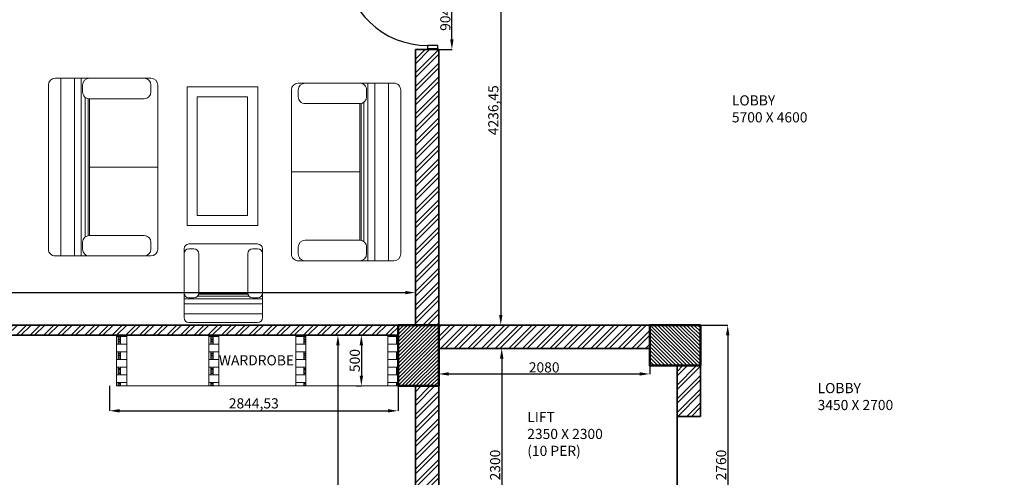
# Model space of a CAD drawing. Units: millimetres. Extents: x -3326 to 29338, y -16792 to 6002.
# Tile 7 of 21: x 7252 to 16958, y -7951 to -3440. Entities that reach past the tile are written whole.
import ezdxf

# ---------------------------------------------------------------- set-up
doc = ezdxf.new("R2010")
doc.units = ezdxf.units.MM
doc.header["$PDMODE"] = 35
doc.header["$PDSIZE"] = 5
for name, color, linetype, lineweight in [('A-ANNO-DIMS', 2, 'Continuous', 13), ('A-AREA-IDEN', 7, 'Continuous', 18), ('A-COLS', 1, 'Continuous', 50), ('A-COLS-PATT', 251, 'Continuous', 13), ('A-DOOR', 3, 'Continuous', 25), ('A-FLOR-CASE', 30, 'Continuous', 18), ('A-FLOR-CASE-PATT', 252, 'Continuous', 13), ('A-WALL', 7, 'Continuous', 35), ('A-WALL-PATT', 252, 'Continuous', 13), ('furn', 28, 'Continuous', 18), ('txt', 7, 'Continuous', 18)]:
    doc.layers.add(name, color=color, linetype=linetype, lineweight=lineweight)
doc.styles.get("Standard").update_dxf_attribs({"font": 'arial.ttf'})
doc.dimstyles.new('ISO-25', dxfattribs={"dimtxt": 100, "dimasz": 100, "dimexe": 1.25, "dimexo": 0.625, "dimtad": 1, "dimtxsty": 'Standard', "dimcen": 2.5, "dimadec": 0, "dimazin": 0, "dimtfac": 1, "dimtmove": 0, "dimatfit": 3, "dimfxl": 1, "dimarcsym": 0})
pattern_1 = [(45, (-10476.65, 1e-12), (-67.35192, 67.35192), []), (45, (-10431.74, 1e-12), (-67.35192, 67.35192), [])]

# ---------------------------------------------------------------- blocks, each defined once
blk = doc.blocks.new('sofa-29')
at = {"color": 0, "linetype": 'ByBlock'}
for p, q in [((1.2, 0.8), (0, 0.8)), ((0.6, 0.8), (0.6, 0.3)), ((-0.05, 0.05), (-0.05, 0.75)), ((-0.05, 0.05), (-0.05, 0.75)), ((0, 0.75), (0.05, 0.75)), ((1.2, 0.75), (1.15, 0.75)), ((1.25, 0.05), (1.25, 0.75)), ((0.1, 0.3), (0.1, 0.7)), ((1.1, 0.3), (1.1, 0.7)), ((1.1, 0.29), (0.099, 0.29)), ((1.1, 0.3), (0.1, 0.3)), ((1.25, 0.24), (-0.05, 0.24)), ((0, 0.25), (0.05, 0.25)), ((1.11, 0.27), (0.09, 0.27)), ((1.2, 0.25), (1.15, 0.25)), ((1.25, 0.19), (-0.05, 0.19)), ((1.25, 0.09), (-0.05, 0.09)), ((1.2, 0), (0, 0))]:
    blk.add_line(p, q, dxfattribs=at)
for centre, start, end in [((0, 0.75), 90, 180), ((1.2, 0.75), 0, 90), ((0, 0.7), 90, 180), ((0.05, 0.7), 0, 90), ((1.15, 0.7), 90, 180), ((1.2, 0.7), 0, 90), ((0, 0.3), 180, 270), ((0.05, 0.3), 270, 0), ((1.15, 0.3), 180, 270), ((1.2, 0.3), 270, 0), ((0, 0.05), 180, 270), ((1.2, 0.05), 270, 0)]:
    blk.add_arc(centre, 0.05, start, end, dxfattribs=at)
blk = doc.blocks.new('sofa-30')
at = {"color": 0, "linetype": 'ByBlock'}
for p, q in [((-0.05, 0.05), (-0.05, 0.75)), ((-0.05, 0.05), (-0.05, 0.75)), ((0.7, 0.8), (0, 0.8)), ((0, 0.75), (0.05, 0.75)), ((0.7, 0.75), (0.65, 0.75)), ((0.75, 0.05), (0.75, 0.75)), ((0.1, 0.3), (0.1, 0.7)), ((0.6, 0.3), (0.6, 0.7)), ((0.75, 0.24), (-0.05, 0.24)), ((0, 0.25), (0.05, 0.25)), ((0.61, 0.27), (0.09, 0.27)), ((0.6, 0.29), (0.099, 0.29)), ((0.6, 0.3), (0.1, 0.3)), ((0.7, 0.25), (0.65, 0.25)), ((0.75, 0.19), (-0.05, 0.19)), ((0.75, 0.09), (-0.05, 0.09)), ((0.7, 0), (0, 0))]:
    blk.add_line(p, q, dxfattribs=at)
for centre, start, end in [((0, 0.75), 90, 180), ((0, 0.7), 90, 180), ((0.05, 0.7), 0, 90), ((0.65, 0.7), 90, 180), ((0.7, 0.75), 0, 90), ((0.7, 0.7), 0, 90), ((0, 0.3), 180, 270), ((0.05, 0.3), 270, 0), ((0.65, 0.3), 180, 270), ((0.7, 0.3), 270, 0), ((0, 0.05), 180, 270), ((0.7, 0.05), 270, 0)]:
    blk.add_arc(centre, 0.05, start, end, dxfattribs=at)
blk = doc.blocks.new('A$C0CE462CD')
for p, q in [((860, 100), (860, 0)), ((860, 0), (893.9, 0))]:
    blk.add_line(p, q)
for points in [[(860, 100), (860, 920), (818.4, 920), (818.4, 100)], [(0, 10), (6.1, 10), (6.1, 90), (0, 90)], [(893.9, 10), (900, 10), (900, 90), (893.9, 90)]]:
    blk.add_lwpolyline(points, close=True)
for points in [[(6.1, 0), (40, 0), (40, 100), (6.1, 100)], [(6.1, 100), (6.1, 0)], [(860, 100), (893.9, 100), (893.9, 0)]]:
    blk.add_lwpolyline(points)
blk.add_arc((859.1, 101.9), 819.1, 92.8508, 180.13091)
blk = doc.blocks.new('*D44')
at = {"layer": 'A-ANNO-DIMS', "color": 0, "lineweight": -2, "transparency": 16777216}
for p, q in [((11382.3, -6681), (11382.3, -6933.5)), ((13462.3, -6681), (13462.3, -6933.5)), ((11482.3, -6932.3), (13362.3, -6932.3))]:
    blk.add_line(p, q, dxfattribs=at)
at = {"layer": 'A-ANNO-DIMS', "color": 0, "transparency": 16777216}
for points in [[(11482.3, -6915.6), (11482.3, -6949), (11382.3, -6932.3)], [(13362.3, -6915.6), (13362.3, -6949), (13462.3, -6932.3)]]:
    blk.add_solid(points, dxfattribs=at)
at = {"layer": 'Defpoints', "color": 0, "transparency": 16777216}
for p in [(11382.3, -6680.4), (13462.3, -6680.4), (13462.3, -6932.3)]:
    blk.add_point(p, dxfattribs=at)
at = {"layer": 'A-ANNO-DIMS', "color": 0, "transparency": 16777216, "insert": (12422.3, -6880.6), "char_height": 100, "attachment_point": 5}
blk.add_mtext('2080', dxfattribs=at)
blk = doc.blocks.new('*D46')
at = {"layer": 'A-ANNO-DIMS', "color": 0, "lineweight": -2, "transparency": 16777216}
for p, q in [((11797.4, -6680.4), (12004.9, -6680.4)), ((12003.7, -6780.4), (12003.7, -8880.4)), ((11797.4, -8980.4), (12004.9, -8980.4))]:
    blk.add_line(p, q, dxfattribs=at)
at = {"layer": 'A-ANNO-DIMS', "color": 0, "transparency": 16777216}
for points in [[(11987, -6780.4), (12020.4, -6780.4), (12003.7, -6680.4)], [(11987, -8880.4), (12020.4, -8880.4), (12003.7, -8980.4)]]:
    blk.add_solid(points, dxfattribs=at)
at = {"layer": 'Defpoints', "color": 0, "transparency": 16777216}
for p in [(11796.7, -6680.4), (11796.7, -8980.4), (12003.7, -8980.4)]:
    blk.add_point(p, dxfattribs=at)
at = {"layer": 'A-ANNO-DIMS', "color": 0, "transparency": 16777216, "insert": (11952, -7830.4), "char_height": 100, "attachment_point": 5, "rotation": 90}
blk.add_mtext('2300', dxfattribs=at)
blk = doc.blocks.new('*D47')
at = {"layer": 'A-ANNO-DIMS', "color": 0, "lineweight": -2, "transparency": 16777216}
for p, q in [((13962.9, -6450.4), (14232.6, -6450.4)), ((14231.3, -6550.4), (14231.3, -9110.4)), ((13962.9, -9210.4), (14232.6, -9210.4))]:
    blk.add_line(p, q, dxfattribs=at)
at = {"layer": 'A-ANNO-DIMS', "color": 0, "transparency": 16777216}
for points in [[(14214.7, -6550.4), (14248, -6550.4), (14231.3, -6450.4)], [(14214.7, -9110.4), (14248, -9110.4), (14231.3, -9210.4)]]:
    blk.add_solid(points, dxfattribs=at)
at = {"layer": 'Defpoints', "color": 0, "transparency": 16777216}
for p in [(13962.3, -6450.4), (13962.3, -9210.4), (14231.3, -9210.4)]:
    blk.add_point(p, dxfattribs=at)
at = {"layer": 'A-ANNO-DIMS', "color": 0, "transparency": 16777216, "insert": (14179.6, -7830.4), "char_height": 100, "attachment_point": 5, "rotation": 90}
blk.add_mtext('2760', dxfattribs=at)
blk = doc.blocks.new('*D49')
at = {"layer": 'A-ANNO-DIMS', "color": 0, "lineweight": -2, "transparency": 16777216}
for p, q in [((12018.3, -2214), (11993.3, -2214)), ((11994.5, -2314), (11994.5, -6350.4)), ((11995.1, -6450.4), (11995.8, -6450.4))]:
    blk.add_line(p, q, dxfattribs=at)
at = {"layer": 'A-ANNO-DIMS', "color": 0, "transparency": 16777216}
for points in [[(11977.9, -2314), (12011.2, -2314), (11994.5, -2214)], [(11977.9, -6350.4), (12011.2, -6350.4), (11994.5, -6450.4)]]:
    blk.add_solid(points, dxfattribs=at)
at = {"layer": 'Defpoints', "color": 0, "transparency": 16777216}
for p in [(12018.9, -2214), (11994.5, -6450.4), (11994.5, -6450.4)]:
    blk.add_point(p, dxfattribs=at)
at = {"layer": 'A-ANNO-DIMS', "color": 0, "transparency": 16777216, "insert": (11933.8, -4332.2), "char_height": 100, "attachment_point": 5, "rotation": 90}
blk.add_mtext('4236,45', dxfattribs=at)
blk = doc.blocks.new('*D59')
at = {"layer": 'A-ANNO-DIMS', "color": 0, "lineweight": -2, "transparency": 16777216}
for p, q in [((10416, -6550.4), (10388, -6550.4)), ((10389.2, -6650.4), (10389.2, -10934)), ((10416, -11034), (10388, -11034))]:
    blk.add_line(p, q, dxfattribs=at)
at = {"layer": 'A-ANNO-DIMS', "color": 0, "transparency": 16777216}
for points in [[(10372.6, -6650.4), (10405.9, -6650.4), (10389.2, -6550.4)], [(10372.6, -10934), (10405.9, -10934), (10389.2, -11034)]]:
    blk.add_solid(points, dxfattribs=at)
at = {"layer": 'Defpoints', "color": 0, "transparency": 16777216}
for p in [(10416.6, -6550.4), (10389.2, -11034), (10416.6, -11034)]:
    blk.add_point(p, dxfattribs=at)
at = {"layer": 'A-ANNO-DIMS', "color": 0, "transparency": 16777216, "insert": (10328.5, -8792.2), "char_height": 100, "attachment_point": 5, "rotation": 90}
blk.add_mtext('4483,55', dxfattribs=at)
blk = doc.blocks.new('*D60')
at = {"layer": 'A-ANNO-DIMS', "color": 0, "lineweight": -2, "transparency": 16777216}
for p, q in [((8137.8, -7051), (8137.8, -7297.3)), ((10982.3, -7051), (10982.3, -7297.3)), ((8237.8, -7296), (10882.3, -7296))]:
    blk.add_line(p, q, dxfattribs=at)
at = {"layer": 'A-ANNO-DIMS', "color": 0, "transparency": 16777216}
for points in [[(8237.8, -7279.3), (8237.8, -7312.7), (8137.8, -7296)], [(10882.3, -7279.3), (10882.3, -7312.7), (10982.3, -7296)]]:
    blk.add_solid(points, dxfattribs=at)
at = {"layer": 'Defpoints', "color": 0, "transparency": 16777216}
for p in [(8137.8, -7050.4), (10982.3, -7050.4), (10982.3, -7296)]:
    blk.add_point(p, dxfattribs=at)
at = {"layer": 'A-ANNO-DIMS', "color": 0, "transparency": 16777216, "insert": (9560, -7235.3), "char_height": 100, "attachment_point": 5}
blk.add_mtext('2844,53', dxfattribs=at)
blk = doc.blocks.new('*D81')
at = {"layer": 'A-ANNO-DIMS', "color": 0, "lineweight": -2, "transparency": 16777216}
for p, q in [((10567.4, -6550.4), (10621.4, -6550.4)), ((10620.1, -6650.4), (10620.1, -6950.4)), ((10567.4, -7050.4), (10621.4, -7050.4))]:
    blk.add_line(p, q, dxfattribs=at)
at = {"layer": 'A-ANNO-DIMS', "color": 0, "transparency": 16777216}
for points in [[(10603.5, -6650.4), (10636.8, -6650.4), (10620.1, -6550.4)], [(10603.5, -6950.4), (10636.8, -6950.4), (10620.1, -7050.4)]]:
    blk.add_solid(points, dxfattribs=at)
at = {"layer": 'Defpoints', "color": 0, "transparency": 16777216}
for p in [(10566.7, -6550.4), (10566.7, -7050.4), (10620.1, -7050.4)]:
    blk.add_point(p, dxfattribs=at)
at = {"layer": 'A-ANNO-DIMS', "color": 0, "transparency": 16777216, "insert": (10568.5, -6800.4), "char_height": 100, "attachment_point": 5, "rotation": 90}
blk.add_mtext('500', dxfattribs=at)
blk = doc.blocks.new('*D92')
at = {"layer": 'A-ANNO-DIMS', "color": 0, "lineweight": -2, "transparency": 16777216}
for p, q in [((1512.3, -5984.6), (1512.3, -6131.9)), ((1612.3, -6130.6), (11052.3, -6130.6)), ((11152.3, -6130), (11152.3, -6129.4))]:
    blk.add_line(p, q, dxfattribs=at)
at = {"layer": 'A-ANNO-DIMS', "color": 0, "transparency": 16777216}
for points in [[(1612.3, -6113.9), (1612.3, -6147.3), (1512.3, -6130.6)], [(11052.3, -6113.9), (11052.3, -6147.3), (11152.3, -6130.6)]]:
    blk.add_solid(points, dxfattribs=at)
at = {"layer": 'Defpoints', "color": 0, "transparency": 16777216}
for p in [(1512.3, -5984), (11152.3, -6130.6), (11152.3, -6130.6)]:
    blk.add_point(p, dxfattribs=at)
at = {"layer": 'A-ANNO-DIMS', "color": 0, "transparency": 16777216, "insert": (6332.3, -6078.9), "char_height": 100, "attachment_point": 5}
blk.add_mtext('9640', dxfattribs=at)
blk = doc.blocks.new('TABLE-COFFEE')
for points in [[(0, 1368.6), (695.8, 1368.6), (695.8, 0), (0, 0)], [(100, 1268.6), (595.8, 1268.6), (595.8, 100), (100, 100)]]:
    blk.add_lwpolyline(points, close=True)
blk = doc.blocks.new('*D196')
at = {"layer": 'A-ANNO-DIMS', "color": 0, "lineweight": -2, "transparency": 16777216}
for p, q in [((11374.5, -2830.4), (11513.7, -2830.4)), ((11512.5, -3634.1), (11512.5, -2930.4)), ((11374.5, -3734.1), (11513.7, -3734.1))]:
    blk.add_line(p, q, dxfattribs=at)
at = {"layer": 'A-ANNO-DIMS', "color": 0, "transparency": 16777216}
for points in [[(11495.8, -2930.4), (11529.1, -2930.4), (11512.5, -2830.4)], [(11495.8, -3634.1), (11529.1, -3634.1), (11512.5, -3734.1)]]:
    blk.add_solid(points, dxfattribs=at)
at = {"layer": 'Defpoints', "color": 0, "transparency": 16777216}
for p in [(11373.9, -2830.4), (11512.5, -2830.4), (11373.9, -3734.1)]:
    blk.add_point(p, dxfattribs=at)
at = {"layer": 'A-ANNO-DIMS', "color": 0, "transparency": 16777216, "insert": (11460.8, -3282.2), "char_height": 100, "attachment_point": 5, "rotation": 90}
blk.add_mtext('904 TYP.', dxfattribs=at)

msp = doc.modelspace()

# ---------------------------------------------------------------- hatches: boundary and pattern name
at = {"layer": 'A-COLS-PATT'}
h = msp.add_hatch(dxfattribs=at)
h.set_pattern_fill('ANSI31', color=256, scale=8)
h.set_pattern_definition([(45, (-30739, 156.603), (-17.960512, 17.960512), [])])
h.paths.add_polyline_path([(10982.301, -7050.401), (11382.301, -7050.401), (11382.301, -6450.401), (10982.301, -6450.401)])
h = msp.add_hatch(dxfattribs=at)
h.set_pattern_fill('ANSI31', color=256, scale=8, angle=-90)
h.set_pattern_definition([(315, (19175.939, 38165.31), (17.960512, 17.960512), [])])
h.paths.add_polyline_path([(13962.301, -6450.401), (13462.301, -6450.401), (13462.301, -6850.401), (13962.301, -6850.401)])
at = {"layer": 'A-FLOR-CASE-PATT'}
h = msp.add_hatch(dxfattribs=at)
h.set_pattern_fill('BRSTONE', color=256, scale=9)
h.set_pattern_definition([(0, (-10476.645, 1e-12), (0, 75.438), []), (90, (-10270.9, 1e-12), (-114.3, 75.438), [75.438, -75.438]), (90, (-10293.77, 1e-12), (-114.3, 75.438), [75.438, -75.438]), (0, (-10270.905, 12.57), (114.3, 75.438), [-205.74, 22.86]), (0, (-10270.905, 25.146), (114.3, 75.438), [-205.74, 22.86]), (0, (-10270.905, 37.72), (114.3, 75.438), [-205.74, 22.86]), (0, (-10270.905, 50.29), (114.3, 75.438), [-205.74, 22.86]), (0, (-10270.905, 62.865), (114.3, 75.438), [-205.74, 22.86])])
h.paths.add_polyline_path([(8307.301, -6550.401), (8207.301, -6550.401), (8207.301, -7050.401), (8307.301, -7050.401)])
h.paths.add_polyline_path([(9215.634, -6550.401), (9115.634, -6550.401), (9115.634, -7050.401), (9215.634, -7050.401)])
h.paths.add_polyline_path([(10073.967, -6550.401), (9973.967, -6550.401), (9973.967, -7050.401), (10073.967, -7050.401)])
h.paths.add_polyline_path([(10982.301, -6550.401), (10882.301, -6550.401), (10882.301, -7050.401), (10982.301, -7050.401)])
at = {"layer": 'A-WALL-PATT'}
h = msp.add_hatch(dxfattribs=at)
h.set_pattern_fill('ANSI32', color=256, scale=10)
h.set_pattern_definition(pattern_1)
h.paths.add_polyline_path([(12212.301, -1983.952), (11640.861, -1983.952), (11640.861, -2213.952), (12212.301, -2213.952)])
h.paths.add_polyline_path([(14712.301, -1983.952), (14012.301, -1983.952), (14012.301, -2213.952), (14712.301, -2213.952)])
h.paths.add_polyline_path([(17012.301, -1983.952), (16512.301, -1983.952), (16512.301, -2213.952), (17012.301, -2213.952)])
h.paths.add_polyline_path([(11382.301, -2383.952), (11040.861, -2383.952), (7302.301, -2383.952), (7302.301, -1935.766), (7217.026, -1935.766), (7202.301, -1933.952), (7202.301, -2483.952), (7302.301, -2483.952), (11152.301, -2483.952), (11152.301, -2833.952), (11283.549, -2833.952), (11283.549, -2830.395), (11363.875, -2830.395), (11382.301, -2833.952)])
h.paths.add_polyline_path([(11382.301, -3733.952), (11363.875, -3733.952), (11363.875, -3734.058), (11283.549, -3734.058), (11152.301, -3733.952), (11152.301, -6450.401), (11382.301, -6450.401)])
h.paths.add_polyline_path([(13462.301, -6450.401), (12606.738, -6450.401), (11382.301, -6450.401), (11382.301, -6680.401), (12606.738, -6680.401), (13462.301, -6680.401)])
h.paths.add_polyline_path([(11382.301, -7050.401), (11152.301, -7050.401), (11152.301, -8810.401), (11382.301, -8810.401)])
h.paths.add_polyline_path([(13462.301, -8980.401), (11751.174, -8980.401), (11751.174, -9210.401), (13462.301, -9210.401)])
h.paths.add_polyline_path([(13962.301, -6850.401), (13732.301, -6850.401), (13732.301, -7350.401), (13962.301, -7350.401)])
h.paths.add_polyline_path([(13962.301, -8309.482), (13732.301, -8309.482), (13732.301, -8809.482), (13962.301, -8809.482)])
h.paths.add_polyline_path([(15712.301, -12533.952), (12902.301, -12533.952), (12902.301, -12763.952), (15712.301, -12763.952)])
h.paths.add_polyline_path([(11508.301, -9211.585), (11382.301, -9211.585), (11152.301, -9211.585), (11152.301, -11033.952), (10952.301, -11033.952), (10952.301, -11263.952), (11152.301, -11263.952), (11152.301, -12361.585), (11508.301, -12361.585)])
h.paths.add_polyline_path([(12002.301, -12533.952), (11902.301, -12533.952), (11902.301, -12761.585), (11152.301, -12761.585), (11152.301, -12763.952), (11902.301, -12763.952), (12002.301, -12763.952)])
h.paths.add_polyline_path([(17112.301, -12533.952), (16912.301, -12533.952), (16912.301, -12763.952), (17112.301, -12763.952)])
h.paths.add_polyline_path([(11382.301, 3596.048), (11152.301, 3596.048), (11152.301, 2096.048), (11382.301, 2096.048)])
h.paths.add_polyline_path([(11382.301, 1496.048), (11152.301, 1496.048), (11152.301, -1983.952), (11382.301, -1983.952)])
h = msp.add_hatch(dxfattribs=at)
h.set_pattern_fill('ANSI32', color=256, scale=10)
h.set_pattern_definition(pattern_1)
h.paths.add_polyline_path([(7302.301, -11263.952), (7902.301, -11263.952), (7902.301, -11033.952), (7302.301, -11033.952), (7302.301, -8110.991), (7202.301, -8110.991), (7202.301, -11033.952), (6672.301, -11033.952), (6672.301, -11263.952), (7072.301, -11263.952), (7072.301, -12763.952), (7302.301, -12763.952)])
h.paths.add_polyline_path([(9152.301, -11033.952), (8802.301, -11033.952), (8802.301, -11044.19), (8802.545, -11044.19), (8802.545, -11124.19), (8802.301, -11263.952), (9152.301, -11263.952)])
h.paths.add_polyline_path([(3712.301, -8110.991), (3612.301, -8110.991), (3612.301, -11033.952), (3282.301, -11033.952), (3282.301, -11263.952), (3612.301, -11263.952), (3612.301, -12763.952), (3842.301, -12763.952), (3842.301, -11263.952), (4092.301, -11263.952), (4092.301, -11033.952), (3842.301, -11033.952), (3712.301, -11033.952)])
h.paths.add_polyline_path([(5172.301, -11033.952), (4692.301, -11033.952), (4692.301, -11263.952), (5172.301, -11263.952)])
h.paths.add_polyline_path([(6072.301, -11033.952), (5572.301, -11033.952), (5572.301, -11263.952), (6072.301, -11263.952)])
h.paths.add_polyline_path([(6072.301, -11263.952), (5972.301, -11263.952), (5972.301, -11663.952), (6072.301, -11663.952)])
h.paths.add_polyline_path([(4792.301, -11263.952), (4692.301, -11263.952), (4692.301, -11663.952), (4792.301, -11663.952)])
h.paths.add_polyline_path([(6402.301, -8110.991), (6272.301, -8110.991), (5572.301, -8110.991), (5572.301, -7200.401), (5342.301, -7200.401), (5342.301, -8110.991), (4642.301, -8110.991), (4512.301, -8110.991), (4512.301, -8210.991), (4642.301, -8210.991), (5342.301, -8210.991), (5342.301, -10513.952), (5572.301, -10513.952), (5572.301, -8210.991), (6272.301, -8210.991), (6402.301, -8210.991)])
h.paths.add_polyline_path([(232.301, -11033.952), (-217.699, -11033.952), (-217.699, -11263.952), (232.301, -11263.952)])
h.paths.add_polyline_path([(1482.301, -11033.952), (1132.301, -11033.952), (1132.301, -11044.8), (1132.987, -11044.8), (1132.987, -11124.8), (1132.301, -11263.952), (1482.301, -11263.952)])
h.paths.add_polyline_path([(-387.699, -11263.952), (-617.699, -11263.952), (-617.699, -12763.952), (-438.882, -12763.952), (-387.699, -12763.952)])
h.paths.add_polyline_path([(-387.699, -7150.401), (-215.519, -7150.401), (-215.519, -7050.401), (-617.699, -7050.401), (-617.699, -10763.952), (-387.699, -10763.952)])
h.paths.add_polyline_path([(1512.301, -5983.952), (1282.301, -5983.952), (1282.301, -6450.401), (-215.519, -6450.401), (-215.519, -6550.401), (4073.51, -6550.401), (4073.51, -6450.401), (1512.301, -6450.401)])
h.paths.add_polyline_path([(5773.51, -6450.401), (5573.51, -6450.401), (5573.51, -6550.401), (5773.51, -6550.401)])
h.paths.add_polyline_path([(5173.51, -6450.401), (4973.51, -6450.401), (4973.51, -6550.401), (5173.51, -6550.401)])
h.paths.add_polyline_path([(10982.301, -6450.401), (6673.51, -6450.401), (6673.51, -6550.401), (10982.301, -6550.401)])

# ---------------------------------------------------------------- linework, layer by layer
at = {"layer": 'A-COLS'}
for points in [[(10982.301, -6450.401), (11382.301, -6450.401), (11382.301, -7050.401), (10982.301, -7050.401)], [(13962.301, -6450.401), (13962.301, -6850.401), (13462.301, -6850.401), (13462.301, -6450.401)]]:
    msp.add_lwpolyline(points, close=True, dxfattribs=at)
at = {"layer": 'A-FLOR-CASE'}
for p, q in [((8207.301, -7050.401), (8207.301, -6550.401)), ((8307.301, -7050.401), (8307.301, -6550.401)), ((9115.634, -7050.401), (9115.634, -6550.401)), ((9215.634, -7050.401), (9215.634, -6550.401)), ((9973.967, -7050.401), (9973.967, -6550.401)), ((10073.967, -7050.401), (10073.967, -6550.401)), ((10882.301, -6550.401), (10882.301, -7050.401)), ((8307.301, -7050.401), (8207.301, -7050.401)), ((10882.301, -7050.401), (8307.301, -7050.401)), ((10982.301, -7050.401), (10882.301, -7050.401))]:
    msp.add_line(p, q, dxfattribs=at)
at = {"layer": 'A-WALL'}
for p, q in [((11382.301, -3733.952), (11152.301, -3733.952)), ((11152.301, -3733.952), (11152.301, -6450.401)), ((11382.301, -3733.952), (11382.301, -8810.401)), ((10982.301, -6450.401), (6673.51, -6450.401)), ((12606.738, -6450.401), (11382.301, -6450.401)), ((12606.738, -6450.401), (13732.301, -6450.401)), ((13732.301, -6450.401), (13962.301, -6450.401)), ((13962.301, -6450.401), (13962.301, -7350.401)), ((10982.301, -6550.401), (6673.51, -6550.401)), ((12606.738, -6680.401), (11382.301, -6680.401)), ((12606.738, -6680.401), (13462.301, -6680.401)), ((13732.301, -6850.401), (13732.301, -8809.482)), ((11152.301, -7050.401), (11152.301, -9211.585)), ((13732.301, -7350.401), (13962.301, -7350.401))]:
    msp.add_line(p, q, dxfattribs=at)

# ---------------------------------------------------------------- block references
at = {"layer": 'A-DOOR', "xscale": 1.004070386304363, "yscale": 1.004070386304363, "zscale": 1.004070386304363, "rotation": 90.00000000000003}
msp.add_blockref('A$C0CE462CD', (11373.915, -3734.058), dxfattribs=at)
at = {"layer": 'furn', "xscale": 1347.213545272558, "yscale": 1347.213545272558, "zscale": 1347.213545272558}
for p, rotation in [((7535.343, -4085.413), 270), ((11008.621, -5749.701), 89.99999999999999)]:
    msp.add_blockref('sofa-29', p, dxfattribs=dict(at, rotation=rotation))
at = {"layer": 'furn'}
msp.add_blockref('TABLE-COFFEE', (8902.914, -5468.994), dxfattribs=at)
at = {"layer": 'furn', "xscale": 967.7745060020527, "yscale": 967.7745060020527, "zscale": 967.7745060020527}
msp.add_blockref('sofa-30', (8920.317, -6425.45), dxfattribs=at)

# ---------------------------------------------------------------- texts
at = {"layer": 'A-AREA-IDEN', "char_height": 100, "attachment_point": 1}
for s, width, insert in [('LOBBY\\P5700 X 4600', 2574.25425, (14272.623, -4185.764)), ('LOBBY\\P3450 X 2700', 1744.80742, (15117.737, -7021.978)), ('LIFT\\P2350 X 2300\\P(10 PER)', 1113.4107, (12255.557, -7307.197))]:
    msp.add_mtext_dynamic_manual_height_columns(s, width=width, gutter_width=12.5, heights=[0], dxfattribs=dict(at, insert=insert))
at = {"layer": 'txt', "insert": (9215.634, -6747.751), "char_height": 100, "attachment_point": 1}
msp.add_mtext_dynamic_manual_height_columns('WARDROBE', width=1168.90663, gutter_width=12.5, heights=[0], dxfattribs=at)

# ---------------------------------------------------------------- dimensions: what is measured, and where the dimension line sits
at = {"layer": 'A-ANNO-DIMS'}
for base, p1, p2, picture, middle in [((11994.519, -6450.401), (12018.923, -2213.952), (11994.519, -6450.401), '*D49', (11933.799, -4332.177)), ((14231.319, -9210.401), (13962.301, -6450.401), (13962.301, -9210.401), '*D47', (14179.637, -7830.401)), ((10389.237, -11033.952), (10416.582, -6550.401), (10416.582, -11033.952), '*D59', (10328.517, -8792.177)), ((10620.146, -7050.401), (10566.743, -6550.401), (10566.743, -7050.401), '*D81', (10568.464, -6800.401)), ((12003.695, -8980.401), (11796.744, -6680.401), (11796.744, -8980.401), '*D46', (11951.978, -7830.401))]:
    dim = msp.add_linear_dim(base=base, p1=p1, p2=p2, angle=90, dimstyle='ISO-25', override={"dimclrd": 0, "dimclre": 0, "dimclrt": 0}, dxfattribs=at)
    dim.commit()
    dim.dimension.update_dxf_attribs({"geometry": picture, "text_midpoint": middle})
dim = msp.add_linear_dim(base=(11512.477, -2830.395), p1=(11373.915, -3734.058), p2=(11373.915, -2830.395), angle=90, text='<> TYP.', dimstyle='ISO-25', override={"dimdec": 0, "dimlfac": 1, "dimrnd": 0, "dimzin": 0, "dimdsep": 46, "dimlunit": 2}, dxfattribs=at)
dim.commit()
dim.dimension.update_dxf_attribs({"geometry": '*D196', "text_midpoint": (11460.795, -3282.227)})
for base, p1, p2, picture, middle in [((11152.301, -6130.603), (1512.301, -5983.952), (11152.301, -6130.603), '*D92', (6332.301, -6078.921)), ((13462.301, -6932.296), (11382.301, -6680.401), (13462.301, -6680.401), '*D44', (12422.301, -6880.614)), ((10982.301, -7296.014), (8137.771, -7050.401), (10982.301, -7050.401), '*D60', (9560.036, -7235.294))]:
    dim = msp.add_linear_dim(base=base, p1=p1, p2=p2, dimstyle='ISO-25', override={"dimclrd": 0, "dimclre": 0, "dimclrt": 0}, dxfattribs=at)
    dim.commit()
    dim.dimension.update_dxf_attribs({"geometry": picture, "text_midpoint": middle})

doc.saveas('drawing.dxf')
